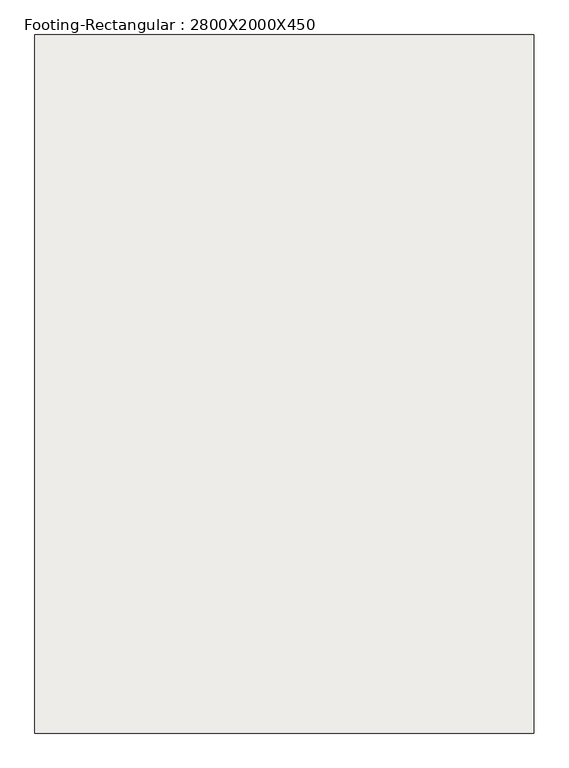
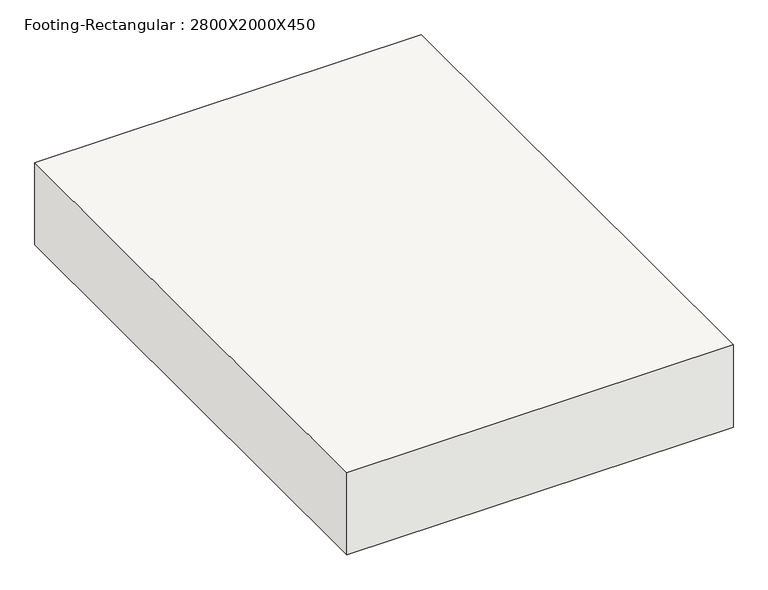
"""IFC4 building model written with IfcOpenShell, lengths in millimetres: slab geometry, Footing-Rectangular : 2800X2000X450."""

from ifc_helpers import new_model, si_unit, frame, origin, place, context, project, spatial, polyline, outline, extrude, source, transform, mapped, element, save


def footing_rectangular_2800x2000x450_516ac05f(model_context):
    return source(origin(), model_context, "Body", "SweptSolid", [
        extrude(outline(polyline([(1000.0, 1400.0), (1000.0, -1400.0), (-1000.0, -1400.0), (-1000.0, 1400.0), (1000.0, 1400.0)])), frame((0.0, 0.0, -450.0), z_axis=(0.0, 0.0, 1.0), x_axis=(1.0, 0.0, 0.0)), (0.0, 0.0, 1.0), 450.0),
    ])


if __name__ == "__main__":
    model = new_model("IFC4")
    model_context = context("Model", 3, world=origin())
    ifc_project = project(units=[si_unit("LENGTHUNIT", "METRE", prefix="MILLI")], contexts=[model_context])
    site = spatial("IfcSite", under=ifc_project)
    building = spatial("IfcBuilding", under=site)
    placement = place(None, origin())
    footing_rectangular_2800x2000x450_shape = footing_rectangular_2800x2000x450_516ac05f(model_context)
    element("IfcSlab", 1, ObjectType="Footing-Rectangular : 2800X2000X450", at=placement, inside=building, context=model_context, shape_type="MappedRepresentation", body=[
        mapped(footing_rectangular_2800x2000x450_shape, transform((0.0, 0.0, 0.0), x_axis=(1.0, 0.0, 0.0), y_axis=(0.0, 1.0, 0.0), z_axis=(0.0, 0.0, 1.0))),
    ])
    save(model, "model.ifc")

# Revit data of these elements
# Type "Footing-Rectangular : 2800X2000X450"
#   Width = 6' - 6.74016"
#   Length = 9' - 2.23622"
#   Foundation Thickness = 1' - 5.71654"
#   Structural Material [instance default] = Concrete - Cast-in-Place Concrete
#   Assembly Code = ""
# Element 1 (IfcSlab, "Footing-Rectangular : 2800X2000X450")
#   Materials on its faces: "Concrete - Cast-in-Place Concrete"
# Materials
#   "Concrete - Cast-in-Place Concrete": class "Concrete", colour RGB 192 192 192, transparency 0, Cost = 0
